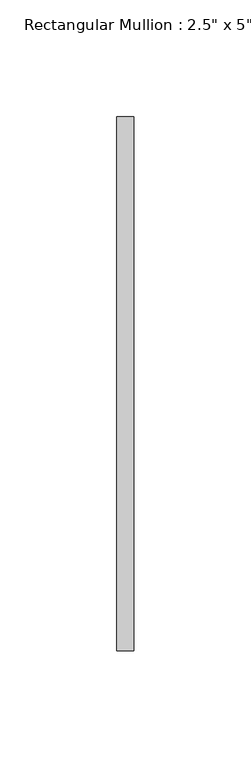
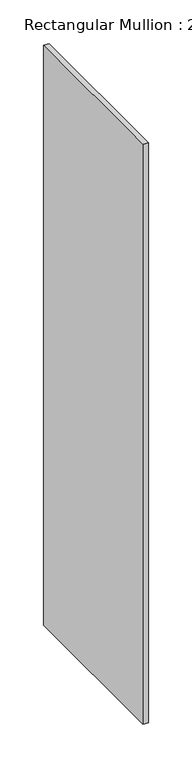
"""IFC4 building model written with IfcOpenShell, lengths in millimetres: member geometry."""

from ifc_helpers import new_model, si_unit, frame, origin, place, context, project, spatial, polyline, outline, extrude, source, transform, mapped, element, save


def member_d66a3bdd(model_context):
    return source(origin(), model_context, "Body", "SweptSolid", [
        extrude(outline(polyline([(0.0, 114.3), (0.0, -114.3), (-7.239, -114.3), (-7.239, 114.3), (0.0, 114.3)])), frame((0.0, 0.0, -812.8), z_axis=(0.0, 0.0, 1.0), x_axis=(1.0, 0.0, 0.0)), (0.0, 0.0, 1.0), 812.8),
    ])


if __name__ == "__main__":
    model = new_model("IFC4")
    model_context = context("Model", 3, world=origin())
    ifc_project = project(units=[si_unit("LENGTHUNIT", "METRE", prefix="MILLI")], contexts=[model_context])
    site = spatial("IfcSite", under=ifc_project)
    building = spatial("IfcBuilding", under=site)
    placement = place(None, origin())
    member_shape = member_d66a3bdd(model_context)
    element("IfcMember", 1, ObjectType="Rectangular Mullion : 2.5\" x 5\" rectangular", at=placement, inside=building, context=model_context, shape_type="MappedRepresentation", body=[
        mapped(member_shape, transform((0.0, 0.0, 0.0), x_axis=(1.0, 0.0, 0.0), y_axis=(0.0, 1.0, 0.0), z_axis=(0.0, 0.0, 1.0))),
    ])
    save(model, "model.ifc")

# Revit data of these elements
# Type "Rectangular Mullion : 2.5\" x 5\" rectangular"
#   built-in parameter 1007304 = 0.75 (stored number, unit not read)
#   built-in parameter 1007301 = 0.011875 (stored number, unit not read)
#   built-in parameter 1007300 = 0.011875 (stored number, unit not read)
# Element 1 (IfcMember, "Rectangular Mullion : 2.5\" x 5\" rectangular")
#   Materials on its faces: "WINDOW GLASS MATERIAL"
# Materials
#   "WINDOW GLASS MATERIAL": class "Generic", colour RGB 120 120 120, transparency 0, Cost = 0
